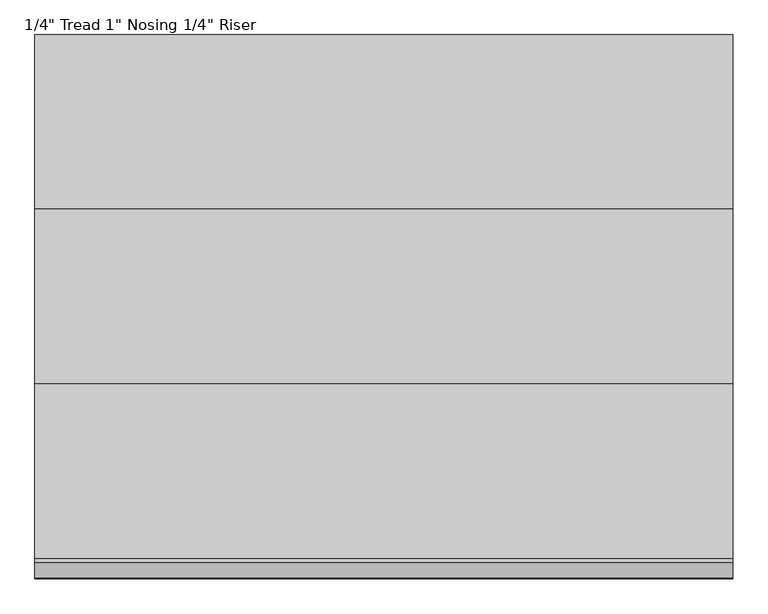
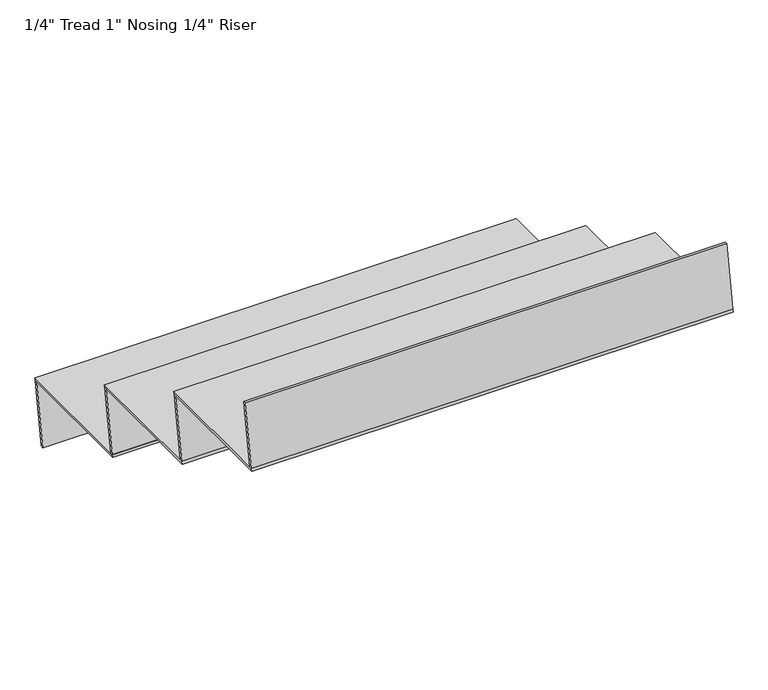
"""IFC4 building model written with IfcOpenShell, lengths in millimetres: stair flight geometry."""

from ifc_helpers import new_model, si_unit, frame, origin, place, context, project, spatial, polyline, outline, extrude, source, transform, mapped, element, save


def stair_flight_a16d44b4(model_context):
    return source(origin(), model_context, "Body", "SweptSolid", [
        extrude(outline(polyline([(5975.7902475, 152.4), (6287.0278379, 152.4), (6285.9695045, 146.05), (5974.7319142, 146.05), (5975.7902475, 152.4)])), frame((-1909.0879185, 0.0, 0.0), z_axis=(1.0, 0.0, 0.0), x_axis=(0.0, 1.0, 0.0)), (0.0, 0.0, 1.0), 1117.6),
        extrude(outline(polyline([(6285.9695045, 146.05), (6261.6278379, 0.0), (6255.1902475, 0.0), (6279.5319142, 146.05), (6285.9695045, 146.05)])), frame((-1909.0879185, 0.0, 0.0), z_axis=(1.0, 0.0, 0.0), x_axis=(0.0, 1.0, 0.0)), (0.0, 0.0, 1.0), 1117.6),
        extrude(outline(polyline([(6006.5695045, 298.45), (5982.2278379, 152.4), (5975.7902475, 152.4), (6000.1319142, 298.45), (6006.5695045, 298.45)])), frame((-1909.0879185, 0.0, 0.0), z_axis=(1.0, 0.0, 0.0), x_axis=(0.0, 1.0, 0.0)), (0.0, 0.0, 1.0), 1117.6),
        extrude(outline(polyline([(5696.3902475, 304.8), (6007.6278379, 304.8), (6006.5695045, 298.45), (5695.3319142, 298.45), (5696.3902475, 304.8)])), frame((-1909.0879185, 0.0, 0.0), z_axis=(1.0, 0.0, 0.0), x_axis=(0.0, 1.0, 0.0)), (0.0, 0.0, 1.0), 1117.6),
        extrude(outline(polyline([(5727.1695045, 450.85), (5702.8278379, 304.8), (5696.3902475, 304.8), (5720.7319142, 450.85), (5727.1695045, 450.85)])), frame((-1909.0879185, 0.0, 0.0), z_axis=(1.0, 0.0, 0.0), x_axis=(0.0, 1.0, 0.0)), (0.0, 0.0, 1.0), 1117.6),
        extrude(outline(polyline([(5447.7695045, 603.25), (5423.4278379, 457.2), (5416.9902475, 457.2), (5441.3319142, 603.25), (5447.7695045, 603.25)])), frame((-1909.0879185, 0.0, 0.0), z_axis=(1.0, 0.0, 0.0), x_axis=(0.0, 1.0, 0.0)), (0.0, 0.0, 1.0), 1117.6),
        extrude(outline(polyline([(5416.9902475, 457.2), (5728.2278379, 457.2), (5727.1695045, 450.85), (5415.9319142, 450.85), (5416.9902475, 457.2)])), frame((-1909.0879185, 0.0, 0.0), z_axis=(1.0, 0.0, 0.0), x_axis=(0.0, 1.0, 0.0)), (0.0, 0.0, 1.0), 1117.6),
    ])


if __name__ == "__main__":
    model = new_model("IFC4")
    model_context = context("Model", 3, world=origin())
    ifc_project = project(units=[si_unit("LENGTHUNIT", "METRE", prefix="MILLI")], contexts=[model_context])
    site = spatial("IfcSite", under=ifc_project)
    building = spatial("IfcBuilding", under=site)
    placement = place(None, origin())
    stair_flight_shape = stair_flight_a16d44b4(model_context)
    element("IfcStairFlight", 1, ObjectType="1/4\" Tread 1\" Nosing 1/4\" Riser", at=placement, inside=building, context=model_context, shape_type="MappedRepresentation", body=[
        mapped(stair_flight_shape, transform((0.0, 0.0, 0.0), x_axis=(1.0, 0.0, 0.0), y_axis=(0.0, 1.0, 0.0), z_axis=(0.0, 0.0, 1.0))),
    ])
    save(model, "model.ifc")

# Revit data of these elements
# Element 1 (IfcStairFlight, "1/4\" Tread 1\" Nosing 1/4\" Riser")
#   Materials on its faces: "Steel, Paint Finish, Dark Gray"
# Materials
#   "Steel, Paint Finish, Dark Gray": class "Metal", colour RGB 89 89 89, transparency 0, Description = "Steel, paint finish, dark gray, glossy", Cost = 0
